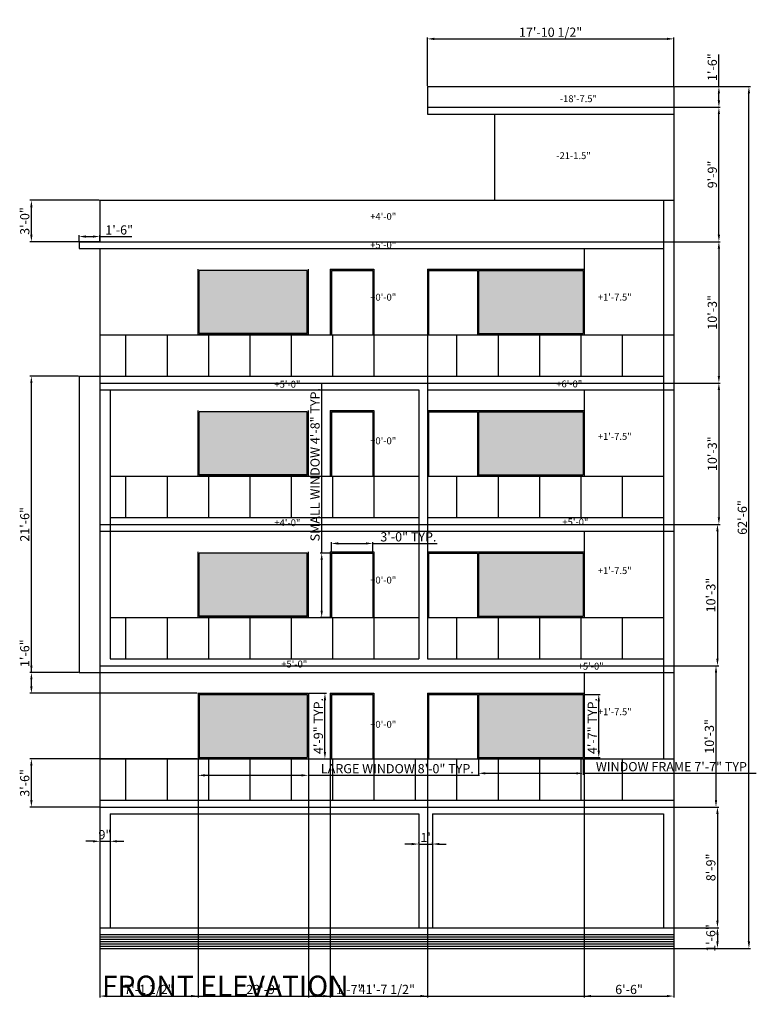
# Model space of a CAD drawing. Units: millimetres. Extents: x 1706 to 5913, y 156 to 1716.
# Tile 21 of 26: x 5272 to 5913, y 191 to 1048. Entities that reach past the tile are written whole.
import ezdxf

# ---------------------------------------------------------------- set-up
doc = ezdxf.new("R2010")
doc.units = ezdxf.units.MM
for name, color, linetype, lineweight in [('A-ANNO-DIMS', 2, 'Continuous', 18), ('A-ANNO-SYMB', 3, 'Continuous', 18), ('A-ANNO-TEXT', 7, 'Continuous', 18), ('A-ELEV', 7, 'Continuous', 25), ('A-ELEV-PATT', 152, 'Continuous', 13)]:
    doc.layers.add(name, color=color, linetype=linetype, lineweight=lineweight)
doc.styles.get("Standard").update_dxf_attribs({"font": 'arial.ttf'})
doc.dimstyles.new('ISO-25', dxfattribs={"dimtxt": 8, "dimasz": 6, "dimexe": 1.25, "dimexo": 0.625, "dimtad": 1, "dimdec": 0, "dimlunit": 3, "dimtxsty": 'Standard', "dimcen": 2.5, "dimadec": 0, "dimazin": 0, "dimtfac": 1, "dimtdec": 0, "dimtmove": 0, "dimatfit": 3, "dimfxl": 1, "dimarcsym": 0})

# ---------------------------------------------------------------- blocks, each defined once
blk = doc.blocks.new('*D195')
at = {"layer": 'A-ANNO-DIMS', "color": 0, "lineweight": -2, "transparency": 16777216}
for p, q in [((5841.64, 362.79), (5880.16, 362.79)), ((5878.91, 356.79), (5878.91, 263.79)), ((5841.64, 257.79), (5880.16, 257.79))]:
    blk.add_line(p, q, dxfattribs=at)
at = {"layer": 'A-ANNO-DIMS', "color": 0, "transparency": 16777216}
for points in [[(5877.91, 356.79), (5879.91, 356.79), (5878.91, 362.79)], [(5877.91, 263.79), (5879.91, 263.79), (5878.91, 257.79)]]:
    blk.add_solid(points, dxfattribs=at)
at = {"layer": 'Defpoints', "color": 0, "transparency": 16777216}
for p in [(5841.01, 362.79), (5841.01, 257.79), (5878.91, 257.79)]:
    blk.add_point(p, dxfattribs=at)
at = {"layer": 'A-ANNO-DIMS', "color": 0, "transparency": 16777216, "insert": (5874.2, 310.29), "char_height": 8, "attachment_point": 5, "rotation": 90}
blk.add_mtext('8\'-9"', dxfattribs=at)
blk = doc.blocks.new('*D196')
at = {"layer": 'A-ANNO-DIMS', "color": 0, "lineweight": -2, "transparency": 16777216}
for p, q in [((5841.64, 485.79), (5878.91, 485.79)), ((5877.66, 368.79), (5877.66, 479.79)), ((5841.64, 362.79), (5878.91, 362.79))]:
    blk.add_line(p, q, dxfattribs=at)
at = {"layer": 'A-ANNO-DIMS', "color": 0, "transparency": 16777216}
for points in [[(5876.66, 479.79), (5878.66, 479.79), (5877.66, 485.79)], [(5876.66, 368.79), (5878.66, 368.79), (5877.66, 362.79)]]:
    blk.add_solid(points, dxfattribs=at)
at = {"layer": 'Defpoints', "color": 0, "transparency": 16777216}
for p in [(5841.01, 485.79), (5877.66, 485.79), (5841.01, 362.79)]:
    blk.add_point(p, dxfattribs=at)
at = {"layer": 'A-ANNO-DIMS', "color": 0, "transparency": 16777216, "insert": (5872.94, 424.29), "char_height": 8, "attachment_point": 5, "rotation": 90}
blk.add_mtext('10\'-3"', dxfattribs=at)
blk = doc.blocks.new('*D201')
at = {"layer": 'A-ANNO-DIMS', "color": 0, "lineweight": -2, "transparency": 16777216}
for p, q in [((5841.64, 608.79), (5880.16, 608.79)), ((5878.91, 602.79), (5878.91, 491.79)), ((5841.64, 485.79), (5880.16, 485.79))]:
    blk.add_line(p, q, dxfattribs=at)
at = {"layer": 'A-ANNO-DIMS', "color": 0, "transparency": 16777216}
for points in [[(5877.91, 602.79), (5879.91, 602.79), (5878.91, 608.79)], [(5877.91, 491.79), (5879.91, 491.79), (5878.91, 485.79)]]:
    blk.add_solid(points, dxfattribs=at)
at = {"layer": 'Defpoints', "color": 0, "transparency": 16777216}
for p in [(5841.01, 608.79), (5841.01, 485.79), (5878.91, 485.79)]:
    blk.add_point(p, dxfattribs=at)
at = {"layer": 'A-ANNO-DIMS', "color": 0, "transparency": 16777216, "insert": (5874.19, 547.29), "char_height": 8, "attachment_point": 5, "rotation": 90}
blk.add_mtext('10\'-3"', dxfattribs=at)
blk = doc.blocks.new('*D202')
at = {"layer": 'A-ANNO-DIMS', "color": 0, "lineweight": -2, "transparency": 16777216}
for p, q in [((5841.64, 731.79), (5881.41, 731.79)), ((5880.16, 725.79), (5880.16, 614.79)), ((5841.64, 608.79), (5881.41, 608.79))]:
    blk.add_line(p, q, dxfattribs=at)
at = {"layer": 'A-ANNO-DIMS', "color": 0, "transparency": 16777216}
for points in [[(5879.16, 725.79), (5881.16, 725.79), (5880.16, 731.79)], [(5879.16, 614.79), (5881.16, 614.79), (5880.16, 608.79)]]:
    blk.add_solid(points, dxfattribs=at)
at = {"layer": 'Defpoints', "color": 0, "transparency": 16777216}
for p in [(5841.01, 731.79), (5841.01, 608.79), (5880.16, 608.79)]:
    blk.add_point(p, dxfattribs=at)
at = {"layer": 'A-ANNO-DIMS', "color": 0, "transparency": 16777216, "insert": (5875.44, 670.29), "char_height": 8, "attachment_point": 5, "rotation": 90}
blk.add_mtext('10\'-3"', dxfattribs=at)
blk = doc.blocks.new('*D203')
at = {"layer": 'A-ANNO-DIMS', "color": 0, "lineweight": -2, "transparency": 16777216}
for p, q in [((5841.64, 854.79), (5881.41, 854.79)), ((5880.16, 848.79), (5880.16, 737.79)), ((5841.64, 731.79), (5881.41, 731.79))]:
    blk.add_line(p, q, dxfattribs=at)
at = {"layer": 'A-ANNO-DIMS', "color": 0, "transparency": 16777216}
for points in [[(5879.16, 848.79), (5881.16, 848.79), (5880.16, 854.79)], [(5879.16, 737.79), (5881.16, 737.79), (5880.16, 731.79)]]:
    blk.add_solid(points, dxfattribs=at)
at = {"layer": 'Defpoints', "color": 0, "transparency": 16777216}
for p in [(5841.01, 854.79), (5841.01, 731.79), (5880.16, 731.79)]:
    blk.add_point(p, dxfattribs=at)
at = {"layer": 'A-ANNO-DIMS', "color": 0, "transparency": 16777216, "insert": (5875.44, 793.29), "char_height": 8, "attachment_point": 5, "rotation": 90}
blk.add_mtext('10\'-3"', dxfattribs=at)
blk = doc.blocks.new('*D204')
at = {"layer": 'A-ANNO-DIMS', "color": 0, "lineweight": -2, "transparency": 16777216}
for p, q in [((5841.64, 971.79), (5881.41, 971.79)), ((5880.16, 860.79), (5880.16, 965.79)), ((5841.64, 854.79), (5881.41, 854.79))]:
    blk.add_line(p, q, dxfattribs=at)
at = {"layer": 'A-ANNO-DIMS', "color": 0, "transparency": 16777216}
for points in [[(5879.16, 965.79), (5881.16, 965.79), (5880.16, 971.79)], [(5879.16, 860.79), (5881.16, 860.79), (5880.16, 854.79)]]:
    blk.add_solid(points, dxfattribs=at)
at = {"layer": 'Defpoints', "color": 0, "transparency": 16777216}
for p in [(5841.01, 971.79), (5880.16, 971.79), (5841.01, 854.79)]:
    blk.add_point(p, dxfattribs=at)
at = {"layer": 'A-ANNO-DIMS', "color": 0, "transparency": 16777216, "insert": (5875.45, 913.29), "char_height": 8, "attachment_point": 5, "rotation": 90}
blk.add_mtext('9\'-9"', dxfattribs=at)
blk = doc.blocks.new('*D205')
at = {"layer": 'A-ANNO-DIMS', "color": 0, "lineweight": -2, "transparency": 16777216}
for p, q in [((5880.16, 989.79), (5880.16, 1017.56)), ((5841.64, 989.79), (5881.41, 989.79)), ((5880.16, 977.79), (5880.16, 983.79)), ((5841.64, 971.79), (5881.41, 971.79))]:
    blk.add_line(p, q, dxfattribs=at)
at = {"layer": 'A-ANNO-DIMS', "color": 0, "transparency": 16777216}
for points in [[(5879.16, 983.79), (5881.16, 983.79), (5880.16, 989.79)], [(5879.16, 977.79), (5881.16, 977.79), (5880.16, 971.79)]]:
    blk.add_solid(points, dxfattribs=at)
at = {"layer": 'Defpoints', "color": 0, "transparency": 16777216}
for p in [(5841.01, 989.79), (5880.16, 989.79), (5841.01, 971.79)]:
    blk.add_point(p, dxfattribs=at)
at = {"layer": 'A-ANNO-DIMS', "color": 0, "transparency": 16777216, "insert": (5875.45, 1006.67), "char_height": 8, "attachment_point": 5, "rotation": 90}
blk.add_mtext('1\'-6"', dxfattribs=at)
blk = doc.blocks.new('*D197')
at = {"layer": 'A-ANNO-DIMS', "color": 0, "lineweight": -2, "transparency": 16777216}
for p, q in [((5323.51, 855.42), (5323.51, 860.51)), ((5329.51, 859.26), (5335.51, 859.26)), ((5341.51, 855.42), (5341.51, 860.51)), ((5341.51, 859.26), (5369.28, 859.26))]:
    blk.add_line(p, q, dxfattribs=at)
at = {"layer": 'A-ANNO-DIMS', "color": 0, "transparency": 16777216}
for points in [[(5329.51, 860.26), (5329.51, 858.26), (5323.51, 859.26)], [(5335.51, 860.26), (5335.51, 858.26), (5341.51, 859.26)]]:
    blk.add_solid(points, dxfattribs=at)
at = {"layer": 'Defpoints', "color": 0, "transparency": 16777216}
for p in [(5341.51, 859.26), (5323.51, 854.79), (5341.51, 854.79)]:
    blk.add_point(p, dxfattribs=at)
at = {"layer": 'A-ANNO-DIMS', "color": 0, "transparency": 16777216, "insert": (5358.4, 863.97), "char_height": 8, "attachment_point": 5}
blk.add_mtext('1\'-6"', dxfattribs=at)
blk = doc.blocks.new('*D198')
at = {"layer": 'A-ANNO-DIMS', "color": 0, "lineweight": -2, "transparency": 16777216}
for p, q in [((5841.64, 257.79), (5880.16, 257.79)), ((5878.91, 251.79), (5878.91, 245.79)), ((5841.64, 239.79), (5880.16, 239.79))]:
    blk.add_line(p, q, dxfattribs=at)
at = {"layer": 'A-ANNO-DIMS', "color": 0, "transparency": 16777216}
for points in [[(5877.91, 251.79), (5879.91, 251.79), (5878.91, 257.79)], [(5877.91, 245.79), (5879.91, 245.79), (5878.91, 239.79)]]:
    blk.add_solid(points, dxfattribs=at)
at = {"layer": 'Defpoints', "color": 0, "transparency": 16777216}
for p in [(5841.01, 257.79), (5841.01, 239.79), (5878.91, 239.79)]:
    blk.add_point(p, dxfattribs=at)
at = {"layer": 'A-ANNO-DIMS', "color": 0, "transparency": 16777216, "insert": (5874.2, 248.79), "char_height": 8, "attachment_point": 5, "rotation": 90}
blk.add_mtext('1\'-6"', dxfattribs=at)
blk = doc.blocks.new('*D199')
at = {"layer": 'A-ANNO-DIMS', "color": 0, "lineweight": -2, "transparency": 16777216}
for p, q in [((5613.01, 330.6), (5607.01, 330.6)), ((5619.01, 331.22), (5619.01, 331.85)), ((5619.01, 330.6), (5631.01, 330.6)), ((5631.01, 331.22), (5631.01, 331.85)), ((5637.01, 330.6), (5643.01, 330.6))]:
    blk.add_line(p, q, dxfattribs=at)
at = {"layer": 'A-ANNO-DIMS', "color": 0, "transparency": 16777216}
for points in [[(5613.01, 331.6), (5613.01, 329.6), (5619.01, 330.6)], [(5637.01, 331.6), (5637.01, 329.6), (5631.01, 330.6)]]:
    blk.add_solid(points, dxfattribs=at)
at = {"layer": 'Defpoints', "color": 0, "transparency": 16777216}
for p in [(5619.01, 330.6), (5631.01, 330.6), (5631.01, 330.6)]:
    blk.add_point(p, dxfattribs=at)
at = {"layer": 'A-ANNO-DIMS', "color": 0, "transparency": 16777216, "insert": (5625.01, 335.24), "char_height": 8, "attachment_point": 5}
blk.add_mtext("1'", dxfattribs=at)
blk = doc.blocks.new('*D200')
at = {"layer": 'A-ANNO-DIMS', "color": 0, "lineweight": -2, "transparency": 16777216}
for p, q in [((5335.51, 332.97), (5329.51, 332.97)), ((5341.51, 332.97), (5350.51, 332.97)), ((5341.51, 332.77), (5341.51, 331.72)), ((5350.51, 332.77), (5350.51, 331.72)), ((5356.51, 332.97), (5362.51, 332.97))]:
    blk.add_line(p, q, dxfattribs=at)
at = {"layer": 'A-ANNO-DIMS', "color": 0, "transparency": 16777216}
for points in [[(5335.51, 333.97), (5335.51, 331.97), (5341.51, 332.97)], [(5356.51, 333.97), (5356.51, 331.97), (5350.51, 332.97)]]:
    blk.add_solid(points, dxfattribs=at)
at = {"layer": 'Defpoints', "color": 0, "transparency": 16777216}
for p in [(5341.51, 333.39), (5350.51, 333.39), (5350.51, 332.97)]:
    blk.add_point(p, dxfattribs=at)
at = {"layer": 'A-ANNO-DIMS', "color": 0, "transparency": 16777216, "insert": (5346.01, 337.68), "char_height": 8, "attachment_point": 5}
blk.add_mtext('9"', dxfattribs=at)
blk = doc.blocks.new('ELEV-WIN-LARGE')
for p, q in [((-1, 56), (95, 56)), ((-1, 56), (-1, -1)), ((0, 55), (94, 55)), ((0, 55), (0, 0)), ((94, 55), (94, 0)), ((95, 56), (95, -1)), ((0, 0), (94, 0))]:
    blk.add_line(p, q)
blk = doc.blocks.new('ELEV-WIN-SMALL')
for p, q in [((0, 56), (36, 56)), ((0, 56), (0, 0)), ((36, 56), (36, 0))]:
    blk.add_line(p, q)
blk = doc.blocks.new('ELEV-WIN-FRAME')
for p, q in [((0, 55), (91, 55)), ((0, 55), (0, 0)), ((91, 55), (91, 0)), ((0, 0), (91, 0))]:
    blk.add_line(p, q)
blk = doc.blocks.new('*D233')
at = {"layer": 'A-ANNO-DIMS', "color": 0, "lineweight": -2, "transparency": 16777216}
for p, q in [((5427.01, 404.17), (5427.01, 389.14)), ((5523.01, 404.17), (5523.01, 389.14)), ((5433.01, 390.39), (5517.01, 390.39)), ((5523.01, 390.39), (5671.81, 390.39))]:
    blk.add_line(p, q, dxfattribs=at)
at = {"layer": 'A-ANNO-DIMS', "color": 0, "transparency": 16777216}
for points in [[(5433.01, 391.39), (5433.01, 389.39), (5427.01, 390.39)], [(5517.01, 391.39), (5517.01, 389.39), (5523.01, 390.39)]]:
    blk.add_solid(points, dxfattribs=at)
at = {"layer": 'Defpoints', "color": 0, "transparency": 16777216}
for p in [(5427.01, 404.79), (5523.01, 404.79), (5523.01, 390.39)]:
    blk.add_point(p, dxfattribs=at)
at = {"layer": 'A-ANNO-DIMS', "color": 0, "transparency": 16777216, "insert": (5600.41, 395.16), "char_height": 8, "attachment_point": 5}
blk.add_mtext('LARGE WINDOW 8\'-0" TYP.', dxfattribs=at)
blk = doc.blocks.new('*D234')
at = {"layer": 'A-ANNO-DIMS', "color": 0, "lineweight": -2, "transparency": 16777216}
for p, q in [((5523.64, 461.79), (5538.66, 461.79)), ((5537.41, 410.79), (5537.41, 455.79)), ((5523.64, 404.79), (5538.66, 404.79))]:
    blk.add_line(p, q, dxfattribs=at)
at = {"layer": 'A-ANNO-DIMS', "color": 0, "transparency": 16777216}
for points in [[(5536.41, 455.79), (5538.41, 455.79), (5537.41, 461.79)], [(5536.41, 410.79), (5538.41, 410.79), (5537.41, 404.79)]]:
    blk.add_solid(points, dxfattribs=at)
at = {"layer": 'Defpoints', "color": 0, "transparency": 16777216}
for p in [(5523.01, 461.79), (5537.41, 461.79), (5523.01, 404.79)]:
    blk.add_point(p, dxfattribs=at)
at = {"layer": 'A-ANNO-DIMS', "color": 0, "transparency": 16777216, "insert": (5532.71, 433.29), "char_height": 8, "attachment_point": 5, "rotation": 90}
blk.add_mtext('4\'-9" TYP.', dxfattribs=at)
blk = doc.blocks.new('*D235')
at = {"layer": 'A-ANNO-DIMS', "color": 0, "lineweight": -2, "transparency": 16777216}
for p, q in [((5534.61, 583.79), (5534.61, 731.66)), ((5542.39, 583.79), (5533.36, 583.79)), ((5534.61, 533.79), (5534.61, 577.79)), ((5542.39, 527.79), (5533.36, 527.79))]:
    blk.add_line(p, q, dxfattribs=at)
at = {"layer": 'A-ANNO-DIMS', "color": 0, "transparency": 16777216}
for points in [[(5533.61, 577.79), (5535.61, 577.79), (5534.61, 583.79)], [(5533.61, 533.79), (5535.61, 533.79), (5534.61, 527.79)]]:
    blk.add_solid(points, dxfattribs=at)
at = {"layer": 'Defpoints', "color": 0, "transparency": 16777216}
for p in [(5534.61, 583.79), (5543.01, 583.79), (5543.01, 527.79)]:
    blk.add_point(p, dxfattribs=at)
at = {"layer": 'A-ANNO-DIMS', "color": 0, "transparency": 16777216, "insert": (5529.85, 660.73), "char_height": 8, "attachment_point": 5, "rotation": 90}
blk.add_mtext('SMALL WINDOW 4\'-8" TYP.', dxfattribs=at)
blk = doc.blocks.new('*D236')
at = {"layer": 'A-ANNO-DIMS', "color": 0, "lineweight": -2, "transparency": 16777216}
for p, q in [((5543.01, 584.42), (5543.01, 593.44)), ((5549.01, 592.19), (5573.01, 592.19)), ((5579.01, 584.42), (5579.01, 593.44)), ((5579.01, 592.19), (5635.02, 592.19))]:
    blk.add_line(p, q, dxfattribs=at)
at = {"layer": 'A-ANNO-DIMS', "color": 0, "transparency": 16777216}
for points in [[(5549.01, 593.19), (5549.01, 591.19), (5543.01, 592.19)], [(5573.01, 593.19), (5573.01, 591.19), (5579.01, 592.19)]]:
    blk.add_solid(points, dxfattribs=at)
at = {"layer": 'Defpoints', "color": 0, "transparency": 16777216}
for p in [(5579.01, 592.19), (5543.01, 583.79), (5579.01, 583.79)]:
    blk.add_point(p, dxfattribs=at)
at = {"layer": 'A-ANNO-DIMS', "color": 0, "transparency": 16777216, "insert": (5610.02, 596.9), "char_height": 8, "attachment_point": 5}
blk.add_mtext('3\'-0" TYP.', dxfattribs=at)
blk = doc.blocks.new('*D237')
at = {"layer": 'A-ANNO-DIMS', "color": 0, "lineweight": -2, "transparency": 16777216}
for p, q in [((5671.01, 405.17), (5671.01, 390.89)), ((5762.01, 405.17), (5762.01, 390.89)), ((5677.01, 392.14), (5756.01, 392.14)), ((5762.01, 392.14), (5912.72, 392.14))]:
    blk.add_line(p, q, dxfattribs=at)
at = {"layer": 'A-ANNO-DIMS', "color": 0, "transparency": 16777216}
for points in [[(5677.01, 393.14), (5677.01, 391.14), (5671.01, 392.14)], [(5756.01, 393.14), (5756.01, 391.14), (5762.01, 392.14)]]:
    blk.add_solid(points, dxfattribs=at)
at = {"layer": 'Defpoints', "color": 0, "transparency": 16777216}
for p in [(5671.01, 405.79), (5762.01, 405.79), (5762.01, 392.14)]:
    blk.add_point(p, dxfattribs=at)
at = {"layer": 'A-ANNO-DIMS', "color": 0, "transparency": 16777216, "insert": (5840.37, 396.91), "char_height": 8, "attachment_point": 5}
blk.add_mtext('WINDOW FRAME 7\'-7" TYP.', dxfattribs=at)
blk = doc.blocks.new('*D238')
at = {"layer": 'A-ANNO-DIMS', "color": 0, "lineweight": -2, "transparency": 16777216}
for p, q in [((5762.64, 460.79), (5776.91, 460.79)), ((5775.66, 411.79), (5775.66, 454.79)), ((5762.64, 405.79), (5776.91, 405.79))]:
    blk.add_line(p, q, dxfattribs=at)
at = {"layer": 'A-ANNO-DIMS', "color": 0, "transparency": 16777216}
for points in [[(5774.66, 454.79), (5776.66, 454.79), (5775.66, 460.79)], [(5774.66, 411.79), (5776.66, 411.79), (5775.66, 405.79)]]:
    blk.add_solid(points, dxfattribs=at)
at = {"layer": 'Defpoints', "color": 0, "transparency": 16777216}
for p in [(5762.01, 460.79), (5775.66, 460.79), (5762.01, 405.79)]:
    blk.add_point(p, dxfattribs=at)
at = {"layer": 'A-ANNO-DIMS', "color": 0, "transparency": 16777216, "insert": (5771.04, 433.29), "char_height": 8, "attachment_point": 5, "rotation": 90}
blk.add_mtext('4\'-7" TYP.', dxfattribs=at)
blk = doc.blocks.new('*D239')
at = {"layer": 'A-ANNO-DIMS', "color": 0, "lineweight": -2, "transparency": 16777216}
for p, q in [((5341.51, 239.17), (5341.51, 197.04)), ((5841.01, 239.17), (5841.01, 197.04)), ((5347.51, 198.29), (5835.01, 198.29))]:
    blk.add_line(p, q, dxfattribs=at)
at = {"layer": 'A-ANNO-DIMS', "color": 0, "transparency": 16777216}
for points in [[(5347.51, 199.29), (5347.51, 197.29), (5341.51, 198.29)], [(5835.01, 199.29), (5835.01, 197.29), (5841.01, 198.29)]]:
    blk.add_solid(points, dxfattribs=at)
at = {"layer": 'Defpoints', "color": 0, "transparency": 16777216}
for p in [(5341.51, 239.79), (5841.01, 239.79), (5841.01, 198.29)]:
    blk.add_point(p, dxfattribs=at)
at = {"layer": 'A-ANNO-DIMS', "color": 0, "transparency": 16777216, "insert": (5591.26, 203.05), "char_height": 8, "attachment_point": 5}
blk.add_mtext('41\'-7 1/2"', dxfattribs=at)
blk = doc.blocks.new('*D240')
at = {"layer": 'A-ANNO-DIMS', "color": 0, "lineweight": -2, "transparency": 16777216}
for p, q in [((5841.64, 989.79), (5907.55, 989.79)), ((5906.3, 245.79), (5906.3, 983.79)), ((5841.64, 239.79), (5907.55, 239.79))]:
    blk.add_line(p, q, dxfattribs=at)
at = {"layer": 'A-ANNO-DIMS', "color": 0, "transparency": 16777216}
for points in [[(5905.3, 983.79), (5907.3, 983.79), (5906.3, 989.79)], [(5905.3, 245.79), (5907.3, 245.79), (5906.3, 239.79)]]:
    blk.add_solid(points, dxfattribs=at)
at = {"layer": 'Defpoints', "color": 0, "transparency": 16777216}
for p in [(5841.01, 989.79), (5906.3, 989.79), (5841.01, 239.79)]:
    blk.add_point(p, dxfattribs=at)
at = {"layer": 'A-ANNO-DIMS', "color": 0, "transparency": 16777216, "insert": (5901.59, 614.79), "char_height": 8, "attachment_point": 5, "rotation": 90}
blk.add_mtext('62\'-6"', dxfattribs=at)
blk = doc.blocks.new('*D241')
at = {"layer": 'A-ANNO-DIMS', "color": 0, "lineweight": -2, "transparency": 16777216}
for p, q in [((5626.51, 990.42), (5626.51, 1032.54)), ((5632.51, 1031.29), (5835.01, 1031.29)), ((5841.01, 990.42), (5841.01, 1032.54))]:
    blk.add_line(p, q, dxfattribs=at)
at = {"layer": 'A-ANNO-DIMS', "color": 0, "transparency": 16777216}
for points in [[(5632.51, 1032.29), (5632.51, 1030.29), (5626.51, 1031.29)], [(5835.01, 1032.29), (5835.01, 1030.29), (5841.01, 1031.29)]]:
    blk.add_solid(points, dxfattribs=at)
at = {"layer": 'Defpoints', "color": 0, "transparency": 16777216}
for p in [(5841.01, 1031.29), (5626.51, 989.79), (5841.01, 989.79)]:
    blk.add_point(p, dxfattribs=at)
at = {"layer": 'A-ANNO-DIMS', "color": 0, "transparency": 16777216, "insert": (5733.76, 1036.05), "char_height": 8, "attachment_point": 5}
blk.add_mtext('17\'-10 1/2"', dxfattribs=at)
blk = doc.blocks.new('*D242')
at = {"layer": 'A-ANNO-DIMS', "color": 0, "lineweight": -2, "transparency": 16777216}
for p, q in [((5341.51, 404.17), (5341.51, 197.04)), ((5427.01, 404.17), (5427.01, 197.04)), ((5347.51, 198.29), (5421.01, 198.29))]:
    blk.add_line(p, q, dxfattribs=at)
at = {"layer": 'A-ANNO-DIMS', "color": 0, "transparency": 16777216}
for points in [[(5347.51, 199.29), (5347.51, 197.29), (5341.51, 198.29)], [(5421.01, 199.29), (5421.01, 197.29), (5427.01, 198.29)]]:
    blk.add_solid(points, dxfattribs=at)
at = {"layer": 'Defpoints', "color": 0, "transparency": 16777216}
for p in [(5341.51, 404.79), (5427.01, 404.79), (5427.01, 198.29)]:
    blk.add_point(p, dxfattribs=at)
at = {"layer": 'A-ANNO-DIMS', "color": 0, "transparency": 16777216, "insert": (5384.26, 203.05), "char_height": 8, "attachment_point": 5}
blk.add_mtext('7\'-1 1/2"', dxfattribs=at)
blk = doc.blocks.new('*D243')
at = {"layer": 'A-ANNO-DIMS', "color": 0, "lineweight": -2, "transparency": 16777216}
for p, q in [((5523.01, 404.17), (5523.01, 197.04)), ((5542.01, 404.17), (5542.01, 197.04)), ((5529.01, 198.29), (5536.01, 198.29)), ((5542.01, 198.29), (5569.78, 198.29))]:
    blk.add_line(p, q, dxfattribs=at)
at = {"layer": 'A-ANNO-DIMS', "color": 0, "transparency": 16777216}
for points in [[(5529.01, 199.29), (5529.01, 197.29), (5523.01, 198.29)], [(5536.01, 199.29), (5536.01, 197.29), (5542.01, 198.29)]]:
    blk.add_solid(points, dxfattribs=at)
at = {"layer": 'Defpoints', "color": 0, "transparency": 16777216}
for p in [(5523.01, 404.79), (5542.01, 404.79), (5542.01, 198.29)]:
    blk.add_point(p, dxfattribs=at)
at = {"layer": 'A-ANNO-DIMS', "color": 0, "transparency": 16777216, "insert": (5558.9, 202.93), "char_height": 8, "attachment_point": 5}
blk.add_mtext('1\'-7"', dxfattribs=at)
blk = doc.blocks.new('*D244')
at = {"layer": 'A-ANNO-DIMS', "color": 0, "lineweight": -2, "transparency": 16777216}
for p, q in [((5341.51, 404.17), (5341.51, 197.04)), ((5626.51, 404.17), (5626.51, 197.04)), ((5347.51, 198.29), (5620.51, 198.29))]:
    blk.add_line(p, q, dxfattribs=at)
at = {"layer": 'A-ANNO-DIMS', "color": 0, "transparency": 16777216}
for points in [[(5347.51, 199.29), (5347.51, 197.29), (5341.51, 198.29)], [(5620.51, 199.29), (5620.51, 197.29), (5626.51, 198.29)]]:
    blk.add_solid(points, dxfattribs=at)
at = {"layer": 'Defpoints', "color": 0, "transparency": 16777216}
for p in [(5341.51, 404.79), (5626.51, 404.79), (5626.51, 198.29)]:
    blk.add_point(p, dxfattribs=at)
at = {"layer": 'A-ANNO-DIMS', "color": 0, "transparency": 16777216, "insert": (5484.01, 203), "char_height": 8, "attachment_point": 5}
blk.add_mtext('23\'-9"', dxfattribs=at)
blk = doc.blocks.new('*D245')
at = {"layer": 'A-ANNO-DIMS', "color": 0, "lineweight": -2, "transparency": 16777216}
for p, q in [((5763.01, 404.17), (5763.01, 197.04)), ((5841.01, 404.17), (5841.01, 197.04)), ((5769.01, 198.29), (5835.01, 198.29))]:
    blk.add_line(p, q, dxfattribs=at)
at = {"layer": 'A-ANNO-DIMS', "color": 0, "transparency": 16777216}
for points in [[(5769.01, 199.29), (5769.01, 197.29), (5763.01, 198.29)], [(5835.01, 199.29), (5835.01, 197.29), (5841.01, 198.29)]]:
    blk.add_solid(points, dxfattribs=at)
at = {"layer": 'Defpoints', "color": 0, "transparency": 16777216}
for p in [(5763.01, 404.79), (5841.01, 404.79), (5841.01, 198.29)]:
    blk.add_point(p, dxfattribs=at)
at = {"layer": 'A-ANNO-DIMS', "color": 0, "transparency": 16777216, "insert": (5802.01, 203), "char_height": 8, "attachment_point": 5}
blk.add_mtext('6\'-6"', dxfattribs=at)
blk = doc.blocks.new('*D246')
at = {"layer": 'A-ANNO-DIMS', "color": 0, "lineweight": -2, "transparency": 16777216}
for p, q in [((5426.39, 404.79), (5280.76, 404.79)), ((5282.01, 368.79), (5282.01, 398.79)), ((5340.89, 362.79), (5280.76, 362.79))]:
    blk.add_line(p, q, dxfattribs=at)
at = {"layer": 'A-ANNO-DIMS', "color": 0, "transparency": 16777216}
for points in [[(5281.01, 398.79), (5283.01, 398.79), (5282.01, 404.79)], [(5281.01, 368.79), (5283.01, 368.79), (5282.01, 362.79)]]:
    blk.add_solid(points, dxfattribs=at)
at = {"layer": 'Defpoints', "color": 0, "transparency": 16777216}
for p in [(5282.01, 404.79), (5427.01, 404.79), (5341.51, 362.79)]:
    blk.add_point(p, dxfattribs=at)
at = {"layer": 'A-ANNO-DIMS', "color": 0, "transparency": 16777216, "insert": (5277.3, 383.79), "char_height": 8, "attachment_point": 5, "rotation": 90}
blk.add_mtext('3\'-6"', dxfattribs=at)
blk = doc.blocks.new('*D247')
at = {"layer": 'A-ANNO-DIMS', "color": 0, "lineweight": -2, "transparency": 16777216}
for p, q in [((5282.01, 479.79), (5282.01, 507.56)), ((5322.89, 479.79), (5280.76, 479.79)), ((5282.01, 467.79), (5282.01, 473.79)), ((5426.39, 461.79), (5280.76, 461.79))]:
    blk.add_line(p, q, dxfattribs=at)
at = {"layer": 'A-ANNO-DIMS', "color": 0, "transparency": 16777216}
for points in [[(5281.01, 473.79), (5283.01, 473.79), (5282.01, 479.79)], [(5281.01, 467.79), (5283.01, 467.79), (5282.01, 461.79)]]:
    blk.add_solid(points, dxfattribs=at)
at = {"layer": 'Defpoints', "color": 0, "transparency": 16777216}
for p in [(5282.01, 479.79), (5323.51, 479.79), (5427.01, 461.79)]:
    blk.add_point(p, dxfattribs=at)
at = {"layer": 'A-ANNO-DIMS', "color": 0, "transparency": 16777216, "insert": (5277.31, 496.67), "char_height": 8, "attachment_point": 5, "rotation": 90}
blk.add_mtext('1\'-6"', dxfattribs=at)
blk = doc.blocks.new('*D248')
at = {"layer": 'A-ANNO-DIMS', "color": 0, "lineweight": -2, "transparency": 16777216}
for p, q in [((5322.89, 737.79), (5280.76, 737.79)), ((5282.01, 485.79), (5282.01, 731.79)), ((5322.89, 479.79), (5280.76, 479.79))]:
    blk.add_line(p, q, dxfattribs=at)
at = {"layer": 'A-ANNO-DIMS', "color": 0, "transparency": 16777216}
for points in [[(5281.01, 731.79), (5283.01, 731.79), (5282.01, 737.79)], [(5281.01, 485.79), (5283.01, 485.79), (5282.01, 479.79)]]:
    blk.add_solid(points, dxfattribs=at)
at = {"layer": 'Defpoints', "color": 0, "transparency": 16777216}
for p in [(5282.01, 737.79), (5323.51, 737.79), (5323.51, 479.79)]:
    blk.add_point(p, dxfattribs=at)
at = {"layer": 'A-ANNO-DIMS', "color": 0, "transparency": 16777216, "insert": (5277.31, 608.79), "char_height": 8, "attachment_point": 5, "rotation": 90}
blk.add_mtext('21\'-6"', dxfattribs=at)
blk = doc.blocks.new('*D249')
at = {"layer": 'A-ANNO-DIMS', "color": 0, "lineweight": -2, "transparency": 16777216}
for p, q in [((5340.89, 890.79), (5280.76, 890.79)), ((5282.01, 860.79), (5282.01, 884.79)), ((5340.89, 854.79), (5280.76, 854.79))]:
    blk.add_line(p, q, dxfattribs=at)
at = {"layer": 'A-ANNO-DIMS', "color": 0, "transparency": 16777216}
for points in [[(5281.01, 884.79), (5283.01, 884.79), (5282.01, 890.79)], [(5281.01, 860.79), (5283.01, 860.79), (5282.01, 854.79)]]:
    blk.add_solid(points, dxfattribs=at)
at = {"layer": 'Defpoints', "color": 0, "transparency": 16777216}
for p in [(5282.01, 890.79), (5341.51, 890.79), (5341.51, 854.79)]:
    blk.add_point(p, dxfattribs=at)
at = {"layer": 'A-ANNO-DIMS', "color": 0, "transparency": 16777216, "insert": (5277.3, 872.79), "char_height": 8, "attachment_point": 5, "rotation": 90}
blk.add_mtext('3\'-0"', dxfattribs=at)

msp = doc.modelspace()

# ---------------------------------------------------------------- hatches: boundary and pattern name
at = {"layer": 'A-ELEV-PATT'}
h = msp.add_hatch(color=256, dxfattribs=at)
h.dxf.hatch_style = 1
h.paths.add_polyline_path([(5522.01, 829.79), (5428.01, 829.79), (5428.01, 774.79), (5522.01, 774.79)])
h = msp.add_hatch(color=256, dxfattribs=at)
h.dxf.hatch_style = 1
h.paths.add_polyline_path([(5762.01, 829.79), (5671.01, 829.79), (5671.01, 774.79), (5762.01, 774.79)])
h = msp.add_hatch(color=256, dxfattribs=at)
h.dxf.hatch_style = 1
h.paths.add_polyline_path([(5522.01, 706.79), (5428.01, 706.79), (5428.01, 651.79), (5522.01, 651.79)])
h = msp.add_hatch(color=256, dxfattribs=at)
h.dxf.hatch_style = 1
h.paths.add_polyline_path([(5762.01, 706.79), (5671.01, 706.79), (5671.01, 651.79), (5762.01, 651.79)])
h = msp.add_hatch(color=256, dxfattribs=at)
h.dxf.hatch_style = 1
h.paths.add_polyline_path([(5522.01, 583.79), (5428.01, 583.79), (5428.01, 528.79), (5522.01, 528.79)])
h = msp.add_hatch(color=256, dxfattribs=at)
h.dxf.hatch_style = 1
h.paths.add_polyline_path([(5762.01, 583.79), (5671.01, 583.79), (5671.01, 528.79), (5762.01, 528.79)])
h = msp.add_hatch(color=256, dxfattribs=at)
h.dxf.hatch_style = 1
h.paths.add_polyline_path([(5522.01, 460.79), (5428.01, 460.79), (5428.01, 405.79), (5522.01, 405.79)])
h = msp.add_hatch(color=256, dxfattribs=at)
h.dxf.hatch_style = 1
h.paths.add_polyline_path([(5762.01, 460.79), (5671.01, 460.79), (5671.01, 405.79), (5762.01, 405.79)])

# ---------------------------------------------------------------- linework, layer by layer
at = {"layer": 'A-ELEV'}
for p, q in [((5626.51, 989.79), (5841.01, 989.79)), ((5626.51, 989.79), (5626.51, 965.79)), ((5841.01, 989.79), (5841.01, 239.79)), ((5626.51, 971.79), (5864.8, 971.79)), ((5626.51, 965.79), (5841.01, 965.79)), ((5684.93, 965.79), (5684.93, 890.79)), ((5341.51, 890.79), (5841.01, 890.79)), ((5341.51, 890.79), (5341.51, 854.79)), ((5832.01, 890.79), (5832.01, 404.79)), ((5323.51, 854.79), (5841.01, 854.79)), ((5323.51, 854.79), (5323.51, 848.79)), ((5323.51, 848.79), (5832.01, 848.79)), ((5341.51, 848.79), (5341.51, 239.79)), ((5763.01, 848.79), (5763.01, 773.79)), ((5542.01, 830.79), (5580.01, 830.79)), ((5542.01, 830.79), (5542.01, 773.79)), ((5580.01, 830.79), (5580.01, 773.79)), ((5626.51, 830.79), (5626.51, 491.79)), ((5626.51, 830.79), (5763.01, 830.79)), ((5627.51, 829.79), (5627.51, 773.79)), ((5627.51, 829.79), (5670.01, 829.79)), ((5670.01, 829.79), (5670.01, 773.79)), ((5341.51, 773.79), (5619.01, 773.79)), ((5364.01, 773.79), (5364.01, 737.79)), ((5400.01, 773.79), (5400.01, 737.79)), ((5436.01, 773.79), (5436.01, 737.79)), ((5472.01, 773.79), (5472.01, 737.79)), ((5508.01, 773.79), (5508.01, 737.79)), ((5544.01, 773.79), (5544.01, 737.79)), ((5580.01, 773.79), (5580.01, 737.79)), ((5619.01, 773.79), (5841.01, 773.79)), ((5652.01, 773.79), (5652.01, 737.79)), ((5688.01, 773.79), (5688.01, 737.79)), ((5724.01, 773.79), (5724.01, 737.79)), ((5760.01, 773.79), (5760.01, 737.79)), ((5796.01, 773.79), (5796.01, 737.79)), ((5323.51, 737.79), (5626.51, 737.79)), ((5323.51, 737.79), (5323.51, 479.79)), ((5626.51, 737.79), (5832.01, 737.79)), ((5341.51, 731.79), (5841.01, 731.79)), ((5341.51, 725.79), (5619.01, 725.79)), ((5350.51, 725.79), (5350.51, 491.79)), ((5619.01, 725.79), (5619.01, 491.79)), ((5626.51, 725.79), (5841.01, 725.79)), ((5763.01, 725.79), (5763.01, 650.79)), ((5542.01, 707.79), (5580.01, 707.79)), ((5542.01, 707.79), (5542.01, 650.79)), ((5580.01, 707.79), (5580.01, 650.79)), ((5626.51, 707.79), (5763.01, 707.79)), ((5627.51, 707.79), (5627.51, 650.79)), ((5627.51, 706.79), (5670.01, 706.79)), ((5670.01, 706.79), (5670.01, 650.79)), ((5350.51, 650.79), (5619.01, 650.79)), ((5364.01, 650.79), (5364.01, 614.79)), ((5400.01, 650.79), (5400.01, 614.79)), ((5436.01, 650.79), (5436.01, 614.79)), ((5472.01, 650.79), (5472.01, 614.79)), ((5508.01, 650.79), (5508.01, 614.79)), ((5544.01, 650.79), (5544.01, 614.79)), ((5580.01, 650.79), (5580.01, 614.79)), ((5626.51, 650.79), (5832.01, 650.79)), ((5652.01, 650.79), (5652.01, 614.79)), ((5688.01, 650.79), (5688.01, 614.79)), ((5724.01, 650.79), (5724.01, 614.79)), ((5760.01, 650.79), (5760.01, 614.79)), ((5796.01, 650.79), (5796.01, 614.79)), ((5341.51, 608.79), (5841.01, 608.79)), ((5350.51, 614.79), (5619.01, 614.79)), ((5626.51, 614.79), (5832.01, 614.79)), ((5341.51, 602.79), (5841.01, 602.79)), ((5763.01, 602.79), (5763.01, 527.79)), ((5542.01, 584.79), (5580.01, 584.79)), ((5542.01, 584.79), (5542.01, 527.79)), ((5580.01, 584.79), (5580.01, 527.79)), ((5626.51, 584.79), (5763.01, 584.79)), ((5627.51, 583.79), (5627.51, 527.79)), ((5627.51, 583.79), (5670.01, 583.79)), ((5670.01, 583.79), (5670.01, 527.79)), ((5350.51, 527.79), (5619.01, 527.79)), ((5364.01, 527.79), (5364.01, 491.79)), ((5400.01, 527.79), (5400.01, 491.79)), ((5436.01, 527.79), (5436.01, 491.79)), ((5472.01, 527.79), (5472.01, 491.79)), ((5508.01, 527.79), (5508.01, 491.79)), ((5544.01, 527.79), (5544.01, 491.79)), ((5580.01, 527.79), (5580.01, 491.79)), ((5626.51, 527.79), (5832.01, 527.79)), ((5652.01, 527.79), (5652.01, 491.79)), ((5688.01, 527.79), (5688.01, 491.79)), ((5724.01, 527.79), (5724.01, 491.79)), ((5760.01, 527.79), (5760.01, 491.79)), ((5796.01, 527.79), (5796.01, 491.79)), ((5350.51, 491.79), (5619.01, 491.79)), ((5626.51, 491.79), (5832.01, 491.79)), ((5341.51, 485.79), (5841.01, 485.79)), ((5323.51, 479.79), (5841.01, 479.79)), ((5763.01, 479.79), (5763.01, 404.79)), ((5542.01, 461.79), (5580.01, 461.79)), ((5542.01, 461.79), (5542.01, 404.79)), ((5580.01, 461.79), (5580.01, 404.79)), ((5626.51, 461.79), (5763.01, 461.79)), ((5626.51, 461.79), (5626.51, 404.79)), ((5626.51, 460.79), (5670.01, 460.79)), ((5627.51, 461.79), (5627.51, 404.79)), ((5631.01, 461.79), (5631.01, 460.79)), ((5670.01, 460.79), (5670.01, 404.79)), ((5341.51, 404.79), (5841.01, 404.79)), ((5364.01, 404.79), (5364.01, 368.79)), ((5400.01, 404.79), (5400.01, 368.79)), ((5436.01, 404.79), (5436.01, 368.79)), ((5472.01, 404.79), (5472.01, 368.79)), ((5508.01, 404.79), (5508.01, 368.79)), ((5544.01, 404.79), (5544.01, 368.79)), ((5580.01, 404.79), (5580.01, 368.79)), ((5616.01, 404.79), (5616.01, 368.79)), ((5652.01, 404.79), (5652.01, 368.79)), ((5688.01, 404.79), (5688.01, 368.79)), ((5724.01, 404.79), (5724.01, 368.79)), ((5760.01, 404.79), (5760.01, 368.79)), ((5796.01, 404.79), (5796.01, 368.79)), ((5341.51, 368.79), (5841.01, 368.79)), ((5341.51, 362.79), (5841.01, 362.79)), ((5350.51, 356.79), (5619.01, 356.79)), ((5350.51, 356.79), (5350.51, 257.79)), ((5619.01, 356.79), (5619.01, 257.79)), ((5631.01, 356.79), (5832.01, 356.79)), ((5631.01, 356.79), (5631.01, 257.79)), ((5832.01, 356.79), (5832.01, 257.79)), ((5341.51, 257.79), (5841.01, 257.79)), ((5341.51, 251.79), (5841.01, 251.79)), ((5341.51, 249.79), (5841.01, 249.79)), ((5341.51, 247.79), (5841.01, 247.79)), ((5341.51, 245.79), (5841.01, 245.79)), ((5341.51, 243.79), (5841.01, 243.79)), ((5341.51, 241.79), (5841.01, 241.79)), ((5341.51, 239.79), (5841.01, 239.79))]:
    msp.add_line(p, q, dxfattribs=at)

# ---------------------------------------------------------------- block references
at = {"layer": 'A-ELEV', "rotation": 180}
for p in [(5522.01, 829.79), (5522.01, 706.79), (5522.01, 583.79)]:
    msp.add_blockref('ELEV-WIN-LARGE', p, dxfattribs=at)
at = {"layer": 'A-ELEV'}
for name, p in [('ELEV-WIN-SMALL', (5543.02, 773.79)), ('ELEV-WIN-FRAME', (5671.02, 774.79)), ('ELEV-WIN-SMALL', (5543.02, 650.79)), ('ELEV-WIN-FRAME', (5671.02, 651.79)), ('ELEV-WIN-SMALL', (5543.02, 527.79)), ('ELEV-WIN-FRAME', (5671.02, 528.79)), ('ELEV-WIN-LARGE', (5428.02, 405.79)), ('ELEV-WIN-SMALL', (5543.02, 404.79)), ('ELEV-WIN-FRAME', (5671.02, 405.79))]:
    msp.add_blockref(name, p, dxfattribs=at)

# ---------------------------------------------------------------- texts
at = {"layer": 'A-ANNO-SYMB', "char_height": 6, "attachment_point": 1}
for s, insert in [('       -18\'-7.5"', (5728.97, 982.22)), ('       +4\'-0"', (5563.98, 879.78)), ('       +5\'-0"', (5563.98, 854.9)), ('       +0\'-0"', (5563.98, 809.45)), ('       +1\'-7.5"', (5762.01, 809.51)), ('       +5\'-0"', (5480.61, 733.73)), ('       +6\'-0"', (5725.82, 734)), ('       +1\'-7.5"', (5762.01, 688.33)), ('       +0\'-0"', (5563.98, 684.49)), ('       +4\'-0"', (5480.61, 613.23)), ('       +5\'-0"', (5731.18, 613.91)), ('       +1\'-7.5"', (5762.01, 571.54)), ('       +0\'-0"', (5563.98, 563.3)), ('       +5\'-0"', (5486.56, 490.23)), ('       +5\'-0"', (5744.46, 488.34)), ('       +1\'-7.5"', (5762.01, 448.72)), ('       +0\'-0"', (5563.98, 437.77))]:
    msp.add_mtext_dynamic_manual_height_columns(s, width=67.9131, gutter_width=12.5, heights=[0], dxfattribs=dict(at, insert=insert))
at = {"layer": 'A-ANNO-TEXT', "attachment_point": 1}
for s, width, insert, char_height in [('       -21-1.5"', 67.9131, (5725.84, 932.66), 6), ('FRONT ELEVATION', 276.4795, (5343.47, 216.07), 18)]:
    msp.add_mtext_dynamic_manual_height_columns(s, width=width, gutter_width=12.5, heights=[0], dxfattribs=dict(at, insert=insert, char_height=char_height))

# ---------------------------------------------------------------- dimensions: what is measured, and where the dimension line sits
at = {"layer": 'A-ANNO-DIMS'}
for base, p1, p2, override, picture, middle in [((5841.01, 1031.29), (5626.51, 989.79), (5841.01, 989.79), {"dimdec": 1, "dimlfac": 1, "dimrnd": 0, "dimzin": 1, "dimdsep": 46, "dimlunit": 4, "dimfrac": 2}, '*D241', (5733.76, 1036.05)), ((5341.51, 859.26), (5323.51, 854.79), (5341.51, 854.79), {"dimclrd": 0, "dimclre": 0, "dimclrt": 0}, '*D197', (5358.4, 863.97)), ((5427.01, 198.29), (5341.51, 404.79), (5427.01, 404.79), {"dimdec": 1, "dimlfac": 1, "dimrnd": 0, "dimzin": 1, "dimdsep": 46, "dimlunit": 4, "dimfrac": 2}, '*D242', (5384.26, 203.05)), ((5626.51, 198.29), (5341.51, 404.79), (5626.51, 404.79), {"dimdec": 1, "dimlfac": 1, "dimrnd": 0, "dimzin": 1, "dimdsep": 46, "dimlunit": 4, "dimfrac": 2}, '*D244', (5484.01, 203)), ((5542.01, 198.29), (5523.01, 404.79), (5542.01, 404.79), {"dimdec": 1, "dimlfac": 1, "dimrnd": 0, "dimzin": 1, "dimdsep": 46, "dimlunit": 4, "dimfrac": 2}, '*D243', (5558.9, 202.93)), ((5841.01, 198.29), (5763.01, 404.79), (5841.01, 404.79), {"dimdec": 1, "dimlfac": 1, "dimrnd": 0, "dimzin": 1, "dimdsep": 46, "dimlunit": 4, "dimfrac": 2}, '*D245', (5802.01, 203)), ((5631.01, 330.6), (5619.01, 330.6), (5631.01, 330.6), {"dimclrd": 0, "dimclre": 0, "dimclrt": 0}, '*D199', (5625.01, 335.24)), ((5841.01, 198.29), (5341.51, 239.79), (5841.01, 239.79), {"dimdec": 1, "dimlfac": 1, "dimrnd": 0, "dimzin": 1, "dimdsep": 46, "dimlunit": 4, "dimfrac": 2}, '*D239', (5591.26, 203.05))]:
    dim = msp.add_linear_dim(base=base, p1=p1, p2=p2, dimstyle='ISO-25', override=override, dxfattribs=at)
    dim.commit()
    dim.dimension.update_dxf_attribs({"geometry": picture, "text_midpoint": middle})
for base, p1, p2, override, picture, middle in [((5880.16, 989.79), (5841.01, 971.79), (5841.01, 989.79), {"dimclrd": 0, "dimclre": 0, "dimclrt": 0}, '*D205', (5875.45, 1006.67)), ((5906.3, 989.79), (5841.01, 239.79), (5841.01, 989.79), {"dimdec": 1, "dimlfac": 1, "dimrnd": 0, "dimzin": 1, "dimdsep": 46, "dimlunit": 4, "dimfrac": 2}, '*D240', (5901.59, 614.79)), ((5880.16, 971.79), (5841.01, 854.79), (5841.01, 971.79), {"dimclrd": 0, "dimclre": 0, "dimclrt": 0}, '*D204', (5875.45, 913.29)), ((5282.01, 890.79), (5341.51, 854.79), (5341.51, 890.79), {"dimdec": 1, "dimlfac": 1, "dimrnd": 0, "dimzin": 1, "dimdsep": 46, "dimlunit": 4, "dimfrac": 2}, '*D249', (5277.3, 872.79)), ((5880.16, 731.79), (5841.01, 854.79), (5841.01, 731.79), {"dimclrd": 0, "dimclre": 0, "dimclrt": 0}, '*D203', (5875.44, 793.29)), ((5282.01, 737.79), (5323.51, 479.79), (5323.51, 737.79), {"dimdec": 1, "dimlfac": 1, "dimrnd": 0, "dimzin": 1, "dimdsep": 46, "dimlunit": 4, "dimfrac": 2}, '*D248', (5277.31, 608.79)), ((5880.16, 608.79), (5841.01, 731.79), (5841.01, 608.79), {"dimclrd": 0, "dimclre": 0, "dimclrt": 0}, '*D202', (5875.44, 670.29)), ((5878.91, 485.79), (5841.01, 608.79), (5841.01, 485.79), {"dimclrd": 0, "dimclre": 0, "dimclrt": 0}, '*D201', (5874.19, 547.29)), ((5282.01, 479.79), (5427.01, 461.79), (5323.51, 479.79), {"dimdec": 1, "dimlfac": 1, "dimrnd": 0, "dimzin": 1, "dimdsep": 46, "dimlunit": 4, "dimfrac": 2}, '*D247', (5277.31, 496.67)), ((5877.66, 485.79), (5841.01, 362.79), (5841.01, 485.79), {"dimclrd": 0, "dimclre": 0, "dimclrt": 0}, '*D196', (5872.94, 424.29)), ((5282.01, 404.79), (5341.51, 362.79), (5427.01, 404.79), {"dimdec": 1, "dimlfac": 1, "dimrnd": 0, "dimzin": 1, "dimdsep": 46, "dimlunit": 4, "dimfrac": 2}, '*D246', (5277.3, 383.79))]:
    dim = msp.add_linear_dim(base=base, p1=p1, p2=p2, angle=90, dimstyle='ISO-25', override=override, dxfattribs=at)
    dim.commit()
    dim.dimension.update_dxf_attribs({"geometry": picture, "text_midpoint": middle})
for base, p1, p2, text, picture, middle in [((5534.61, 583.79), (5543.01, 527.79), (5543.01, 583.79), 'SMALL WINDOW <> TYP.', '*D235', (5529.85, 660.73)), ((5537.41, 461.79), (5523.01, 404.79), (5523.01, 461.79), '<> TYP.', '*D234', (5532.71, 433.29)), ((5775.66, 460.79), (5762.01, 405.79), (5762.01, 460.79), '<> TYP.', '*D238', (5771.04, 433.29))]:
    dim = msp.add_linear_dim(base=base, p1=p1, p2=p2, angle=90, text=text, dimstyle='ISO-25', override={"dimdec": 1, "dimrnd": 0, "dimzin": 1, "dimlunit": 4, "dimfrac": 2}, dxfattribs=at)
    dim.commit()
    dim.dimension.update_dxf_attribs({"geometry": picture, "text_midpoint": middle})
for base, p1, p2, text, picture, middle in [((5579.01, 592.19), (5543.01, 583.79), (5579.01, 583.79), '<> TYP.', '*D236', (5610.02, 596.9)), ((5523.01, 390.39), (5427.01, 404.79), (5523.01, 404.79), 'LARGE WINDOW <> TYP.', '*D233', (5600.41, 395.16)), ((5762.01, 392.14), (5671.01, 405.79), (5762.01, 405.79), 'WINDOW FRAME <> TYP.', '*D237', (5840.37, 396.91))]:
    dim = msp.add_linear_dim(base=base, p1=p1, p2=p2, text=text, dimstyle='ISO-25', override={"dimdec": 1, "dimrnd": 0, "dimzin": 1, "dimlunit": 4, "dimfrac": 2}, dxfattribs=at)
    dim.commit()
    dim.dimension.update_dxf_attribs({"geometry": picture, "text_midpoint": middle})
for base, p1, p2, picture, middle in [((5878.91, 257.79), (5841.01, 362.79), (5841.01, 257.79), '*D195', (5878.91, 310.29)), ((5878.91, 239.79), (5841.01, 257.79), (5841.01, 239.79), '*D198', (5878.91, 248.79))]:
    dim = msp.add_linear_dim(base=base, p1=p1, p2=p2, angle=90, dimstyle='ISO-25', override={"dimclrd": 0, "dimclre": 0, "dimclrt": 0}, dxfattribs=at)
    dim.commit()
    dim.dimension.update_dxf_attribs({"geometry": picture, "text_midpoint": middle, "dimtype": 160})
dim = msp.add_linear_dim(base=(5350.51, 332.97), p1=(5341.51, 333.39), p2=(5350.51, 333.39), dimstyle='ISO-25', override={"dimclrd": 0, "dimclre": 0, "dimclrt": 0}, dxfattribs=at)
dim.commit()
dim.dimension.update_dxf_attribs({"geometry": '*D200', "text_midpoint": (5346.01, 332.97), "dimtype": 160})

doc.saveas('drawing.dxf')
